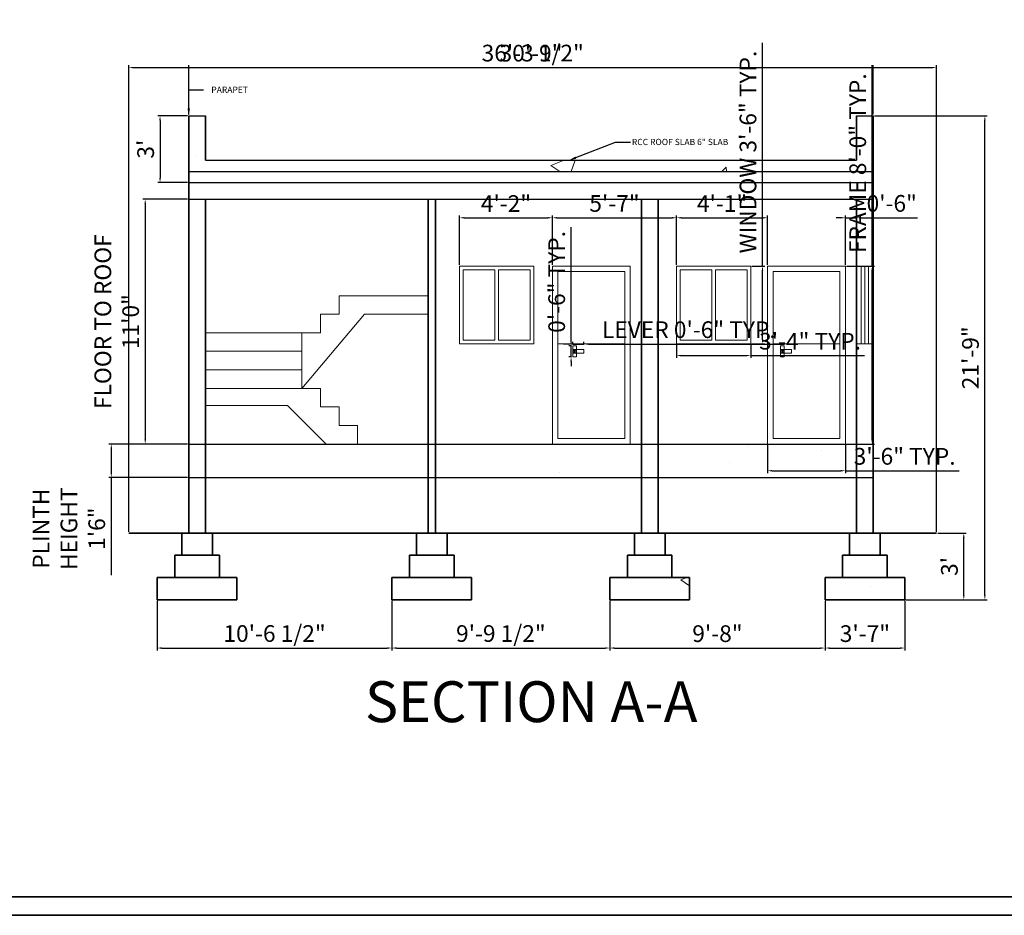
# Model space of a CAD drawing. Units: inches. Extents: x 2413 to 4117, y 1127 to 2321.
# Tile 2 of 5: x 2993 to 3524, y 1127 to 1610. Entities that reach past the tile are written whole.
import ezdxf
from ezdxf import colors
from ezdxf.entities.mleader import LeaderData, LeaderLine
from ezdxf.math import Vec2, Vec3

# ---------------------------------------------------------------- set-up
doc = ezdxf.new("R2010")
doc.units = ezdxf.units.IN
doc.linetypes.add('ACAD_ISO03W100', pattern=[30, 12, -18])
doc.layers.get('Defpoints').update_dxf_attribs({"linetype": 'ACAD_ISO03W100'})
for name, color, linetype, lineweight in [('A-ANNO-DIMS', 2, 'Continuous', 18), ('A-ANNO-TEXT', 7, 'Continuous', 18), ('A-ANNO-TITL', 7, 'Continuous', 30), ('A-ANNO-TTLB', 7, 'Continuous', 35), ('A-DOOR', 3, 'Continuous', 20), ('A-FLOR', 7, 'Continuous', 30), ('A-FLOR-STRS', 3, 'Continuous', 20), ('A-GLAZ', 4, 'Continuous', 18), ('A-ROOF', 7, 'Continuous', 30), ('A-SECT', 7, 'Continuous', 35), ('S-FNDN', 1, 'Continuous', 35), ('S-SECT-PATT', 252, 'Continuous', 13)]:
    doc.layers.add(name, color=color, linetype=linetype, lineweight=lineweight)
doc.styles.get("Standard").update_dxf_attribs({"font": 'arial.ttf'})
doc.dimstyles.new('ISO-25', dxfattribs={"dimtxt": 9, "dimasz": 2.5, "dimexe": 1.25, "dimexo": 0.625, "dimgap": 2, "dimtad": 1, "dimdec": 1, "dimlunit": 4, "dimtxsty": 'Standard', "dimcen": 2.5, "dimazin": 0, "dimtfac": 1, "dimtdec": 1, "dimtmove": 0, "dimatfit": 3, "dimfxl": 1, "dimarcsym": 0})

# ---------------------------------------------------------------- blocks, each defined once
blk = doc.blocks.new('*D1')
at = {"layer": 'A-ANNO-DIMS', "color": 0, "lineweight": -2, "transparency": 16777216}
for p, q in [((3083.32, 1513.03), (3059.22, 1513.03)), ((3060.47, 1510.53), (3060.47, 1383.53)), ((3083.32, 1381.03), (3059.22, 1381.03))]:
    blk.add_line(p, q, dxfattribs=at)
at = {"layer": 'A-ANNO-DIMS', "color": 0, "transparency": 16777216}
for points in [[(3060.06, 1510.53), (3060.89, 1510.53), (3060.47, 1513.03)], [(3060.06, 1383.53), (3060.89, 1383.53), (3060.47, 1381.03)]]:
    blk.add_solid(points, dxfattribs=at)
at = {"layer": 'Defpoints', "color": 0, "transparency": 16777216}
for p in [(3083.95, 1513.03), (3060.47, 1381.03), (3083.95, 1381.03)]:
    blk.add_point(p, dxfattribs=at)
at = {"layer": 'A-ANNO-DIMS', "color": 0, "transparency": 16777216, "insert": (3046.3, 1447.03), "char_height": 9, "attachment_point": 5, "rotation": 90}
blk.add_mtext('FLOOR TO ROOF\\P11\'0"', dxfattribs=at)
blk = doc.blocks.new('*D2')
at = {"layer": 'A-ANNO-DIMS', "color": 0, "lineweight": -2, "transparency": 16777216}
for p, q in [((3083.32, 1558.03), (3067.22, 1558.03)), ((3068.47, 1555.53), (3068.47, 1524.53)), ((3083.32, 1522.03), (3067.22, 1522.03))]:
    blk.add_line(p, q, dxfattribs=at)
at = {"layer": 'A-ANNO-DIMS', "color": 0, "transparency": 16777216}
for points in [[(3068.06, 1555.53), (3068.89, 1555.53), (3068.47, 1558.03)], [(3068.06, 1524.53), (3068.89, 1524.53), (3068.47, 1522.03)]]:
    blk.add_solid(points, dxfattribs=at)
at = {"layer": 'Defpoints', "color": 0, "transparency": 16777216}
for p in [(3083.95, 1558.03), (3068.47, 1522.03), (3083.95, 1522.03)]:
    blk.add_point(p, dxfattribs=at)
at = {"layer": 'A-ANNO-DIMS', "color": 0, "transparency": 16777216, "insert": (3061.87, 1540.03), "char_height": 9, "attachment_point": 5, "rotation": 90}
blk.add_mtext("3'", dxfattribs=at)
blk = doc.blocks.new('*D3')
at = {"layer": 'A-ANNO-DIMS', "color": 0, "lineweight": -2, "transparency": 16777216}
for p, q in [((3083.32, 1381.03), (3040.94, 1381.03)), ((3042.19, 1378.53), (3042.19, 1365.53)), ((3083.32, 1363.03), (3040.94, 1363.03)), ((3042.19, 1363.03), (3042.19, 1310.29))]:
    blk.add_line(p, q, dxfattribs=at)
at = {"layer": 'A-ANNO-DIMS', "color": 0, "transparency": 16777216}
for points in [[(3041.77, 1378.53), (3042.6, 1378.53), (3042.19, 1381.03)], [(3041.77, 1365.53), (3042.6, 1365.53), (3042.19, 1363.03)]]:
    blk.add_solid(points, dxfattribs=at)
at = {"layer": 'Defpoints', "color": 0, "transparency": 16777216}
for p in [(3083.95, 1381.03), (3042.19, 1363.03), (3083.95, 1363.03)]:
    blk.add_point(p, dxfattribs=at)
at = {"layer": 'A-ANNO-DIMS', "color": 0, "transparency": 16777216, "insert": (3020.52, 1335.41), "char_height": 9, "width": 9.6125, "attachment_point": 5, "rotation": 90}
blk.add_mtext('PLINTH HEIGHT \\P1\'6"', dxfattribs=at)
blk = doc.blocks.new('*D4')
at = {"layer": 'A-ANNO-DIMS', "color": 0, "lineweight": -2, "transparency": 16777216}
for p, q in [((3487.74, 1333.03), (3503.01, 1333.03)), ((3501.76, 1299.53), (3501.76, 1330.53)), ((3470.57, 1297.03), (3503.01, 1297.03))]:
    blk.add_line(p, q, dxfattribs=at)
at = {"layer": 'A-ANNO-DIMS', "color": 0, "transparency": 16777216}
for points in [[(3501.34, 1330.53), (3502.17, 1330.53), (3501.76, 1333.03)], [(3501.34, 1299.53), (3502.17, 1299.53), (3501.76, 1297.03)]]:
    blk.add_solid(points, dxfattribs=at)
at = {"layer": 'Defpoints', "color": 0, "transparency": 16777216}
for p in [(3487.11, 1333.03), (3501.76, 1333.03), (3469.95, 1297.03)]:
    blk.add_point(p, dxfattribs=at)
at = {"layer": 'A-ANNO-DIMS', "color": 0, "transparency": 16777216, "insert": (3495.16, 1315.03), "char_height": 9, "attachment_point": 5, "rotation": 90}
blk.add_mtext("3'", dxfattribs=at)
blk = doc.blocks.new('WIN-TWINLIGHT-40x42')
for p, q in [((0, 42), (0, 0)), ((0, 42), (40, 42)), ((2, 40), (19, 40)), ((2, 40), (2, 2)), ((19, 40), (19, 2)), ((21, 40), (21, 2)), ((21, 40), (38, 40)), ((38, 40), (38, 2)), ((40, 42), (40, 0)), ((2, 2), (19, 2)), ((21, 2), (38, 2)), ((0, 0), (40, 0))]:
    blk.add_line(p, q)
blk = doc.blocks.new('DOOR-FRAMED-42x96')
for p, q in [((0, 96), (0, 0)), ((0, 96), (42, 96)), ((42, 96), (42, 0)), ((3, 93), (39, 93)), ((3, 93), (3, 3)), ((39, 93), (39, 3)), ((3, 54), (39, 54)), ((3, 3), (39, 3))]:
    blk.add_line(p, q)
blk = doc.blocks.new('DOOR-LEVER-ELEV')
for p, q in [((0, 6), (0, 0)), ((0, 6), (2, 6)), ((2, 6), (2, 0)), ((0, 4), (6, 4)), ((0, 2), (6, 2)), ((0.18, 3), (1.82, 3)), ((1, 2.18), (1, 3.82)), ((6, 4), (6, 2)), ((0, 0), (2, 0))]:
    blk.add_line(p, q)
blk.add_circle((1, 3), 0.816)
blk = doc.blocks.new('*D26')
at = {"layer": 'A-ANNO-DIMS', "color": 0, "lineweight": -2, "transparency": 16777216}
for p, q in [((3393.25, 1477.03), (3393.25, 1597.42)), ((3387.57, 1477.03), (3394.5, 1477.03)), ((3393.25, 1437.53), (3393.25, 1474.53)), ((3387.57, 1435.03), (3394.5, 1435.03))]:
    blk.add_line(p, q, dxfattribs=at)
at = {"layer": 'A-ANNO-DIMS', "color": 0, "transparency": 16777216}
for points in [[(3392.83, 1474.53), (3393.66, 1474.53), (3393.25, 1477.03)], [(3392.83, 1437.53), (3393.66, 1437.53), (3393.25, 1435.03)]]:
    blk.add_solid(points, dxfattribs=at)
at = {"layer": 'Defpoints', "color": 0, "transparency": 16777216}
for p in [(3386.95, 1477.03), (3393.25, 1477.03), (3386.95, 1435.03)]:
    blk.add_point(p, dxfattribs=at)
at = {"layer": 'A-ANNO-DIMS', "color": 0, "transparency": 16777216, "insert": (3386.59, 1538.48), "char_height": 9, "attachment_point": 5, "rotation": 90}
blk.add_mtext('WINDOW 3\'-6" TYP.', dxfattribs=at)
blk = doc.blocks.new('*D27')
at = {"layer": 'A-ANNO-DIMS', "color": 0, "lineweight": -2, "transparency": 16777216}
for p, q in [((3346.95, 1434.41), (3346.95, 1427.48)), ((3386.95, 1434.41), (3386.95, 1427.48)), ((3349.45, 1428.73), (3384.45, 1428.73)), ((3386.95, 1428.73), (3448.3, 1428.73))]:
    blk.add_line(p, q, dxfattribs=at)
at = {"layer": 'A-ANNO-DIMS', "color": 0, "transparency": 16777216}
for points in [[(3349.45, 1429.15), (3349.45, 1428.32), (3346.95, 1428.73)], [(3384.45, 1429.15), (3384.45, 1428.32), (3386.95, 1428.73)]]:
    blk.add_solid(points, dxfattribs=at)
at = {"layer": 'Defpoints', "color": 0, "transparency": 16777216}
for p in [(3346.95, 1435.03), (3386.95, 1435.03), (3386.95, 1428.73)]:
    blk.add_point(p, dxfattribs=at)
at = {"layer": 'A-ANNO-DIMS', "color": 0, "transparency": 16777216, "insert": (3418.87, 1435.33), "char_height": 9, "attachment_point": 5}
blk.add_mtext('3\'-4" TYP.', dxfattribs=at)
blk = doc.blocks.new('*D28')
at = {"layer": 'A-ANNO-DIMS', "color": 0, "lineweight": -2, "transparency": 16777216}
for p, q in [((3452.35, 1477.03), (3452.35, 1585.38)), ((3438.57, 1477.03), (3453.6, 1477.03)), ((3452.35, 1383.53), (3452.35, 1474.53)), ((3438.57, 1381.03), (3453.6, 1381.03))]:
    blk.add_line(p, q, dxfattribs=at)
at = {"layer": 'A-ANNO-DIMS', "color": 0, "transparency": 16777216}
for points in [[(3451.93, 1474.53), (3452.76, 1474.53), (3452.35, 1477.03)], [(3451.93, 1383.53), (3452.76, 1383.53), (3452.35, 1381.03)]]:
    blk.add_solid(points, dxfattribs=at)
at = {"layer": 'Defpoints', "color": 0, "transparency": 16777216}
for p in [(3437.95, 1477.03), (3452.35, 1477.03), (3437.95, 1381.03)]:
    blk.add_point(p, dxfattribs=at)
at = {"layer": 'A-ANNO-DIMS', "color": 0, "transparency": 16777216, "insert": (3445.75, 1532.46), "char_height": 9, "attachment_point": 5, "rotation": 90}
blk.add_mtext('FRAME 8\'-0" TYP.', dxfattribs=at)
blk = doc.blocks.new('*D29')
at = {"layer": 'A-ANNO-DIMS', "color": 0, "lineweight": -2, "transparency": 16777216}
for p, q in [((3395.95, 1380.41), (3395.95, 1365.38)), ((3437.95, 1380.41), (3437.95, 1365.38)), ((3398.45, 1366.63), (3435.45, 1366.63)), ((3437.95, 1366.63), (3499.3, 1366.63))]:
    blk.add_line(p, q, dxfattribs=at)
at = {"layer": 'A-ANNO-DIMS', "color": 0, "transparency": 16777216}
for points in [[(3398.45, 1367.05), (3398.45, 1366.22), (3395.95, 1366.63)], [(3435.45, 1367.05), (3435.45, 1366.22), (3437.95, 1366.63)]]:
    blk.add_solid(points, dxfattribs=at)
at = {"layer": 'Defpoints', "color": 0, "transparency": 16777216}
for p in [(3395.95, 1381.03), (3437.95, 1381.03), (3437.95, 1366.63)]:
    blk.add_point(p, dxfattribs=at)
at = {"layer": 'A-ANNO-DIMS', "color": 0, "transparency": 16777216, "insert": (3469.87, 1373.23), "char_height": 9, "attachment_point": 5}
blk.add_mtext('3\'-6" TYP.', dxfattribs=at)
blk = doc.blocks.new('*D30')
at = {"layer": 'A-ANNO-DIMS', "color": 0, "lineweight": -2, "transparency": 16777216}
for p, q in [((3288.45, 1434.93), (3285.95, 1434.93)), ((3290.95, 1434.66), (3290.95, 1436.18)), ((3290.95, 1434.93), (3296.95, 1434.93)), ((3296.95, 1434.66), (3296.95, 1436.18)), ((3299.45, 1434.93), (3405.13, 1434.93))]:
    blk.add_line(p, q, dxfattribs=at)
at = {"layer": 'A-ANNO-DIMS', "color": 0, "transparency": 16777216}
for points in [[(3288.45, 1435.35), (3288.45, 1434.52), (3290.95, 1434.93)], [(3299.45, 1435.35), (3299.45, 1434.52), (3296.95, 1434.93)]]:
    blk.add_solid(points, dxfattribs=at)
at = {"layer": 'Defpoints', "color": 0, "transparency": 16777216}
for p in [(3290.95, 1434.03), (3296.95, 1434.93), (3296.95, 1434.03)]:
    blk.add_point(p, dxfattribs=at)
at = {"layer": 'A-ANNO-DIMS', "color": 0, "transparency": 16777216, "insert": (3353.54, 1441.53), "char_height": 9, "attachment_point": 5}
blk.add_mtext('LEVER 0\'-6" TYP.', dxfattribs=at)
blk = doc.blocks.new('*D31')
at = {"layer": 'A-ANNO-DIMS', "color": 0, "lineweight": -2, "transparency": 16777216}
for p, q in [((3290.05, 1436.53), (3290.05, 1497.89)), ((3290.32, 1434.03), (3288.8, 1434.03)), ((3290.05, 1428.03), (3290.05, 1434.03)), ((3290.32, 1428.03), (3288.8, 1428.03)), ((3290.05, 1425.53), (3290.05, 1423.03))]:
    blk.add_line(p, q, dxfattribs=at)
at = {"layer": 'A-ANNO-DIMS', "color": 0, "transparency": 16777216}
for points in [[(3289.63, 1436.53), (3290.46, 1436.53), (3290.05, 1434.03)], [(3289.63, 1425.53), (3290.46, 1425.53), (3290.05, 1428.03)]]:
    blk.add_solid(points, dxfattribs=at)
at = {"layer": 'Defpoints', "color": 0, "transparency": 16777216}
for p in [(3290.05, 1434.03), (3290.95, 1434.03), (3290.95, 1428.03)]:
    blk.add_point(p, dxfattribs=at)
at = {"layer": 'A-ANNO-DIMS', "color": 0, "transparency": 16777216, "insert": (3283.45, 1468.46), "char_height": 9, "attachment_point": 5, "rotation": 90}
blk.add_mtext('0\'-6" TYP.', dxfattribs=at)
blk = doc.blocks.new('*D77')
at = {"layer": 'A-ANNO-DIMS', "color": 0, "lineweight": -2, "transparency": 16777216}
for p, q in [((3051.65, 1333.66), (3051.65, 1585.28)), ((3054.15, 1584.03), (3484.61, 1584.03)), ((3487.11, 1333.66), (3487.11, 1585.28))]:
    blk.add_line(p, q, dxfattribs=at)
at = {"layer": 'A-ANNO-DIMS', "color": 0, "transparency": 16777216}
for points in [[(3054.15, 1584.45), (3054.15, 1583.62), (3051.65, 1584.03)], [(3484.61, 1584.45), (3484.61, 1583.62), (3487.11, 1584.03)]]:
    blk.add_solid(points, dxfattribs=at)
at = {"layer": 'Defpoints', "color": 0, "transparency": 16777216}
for p in [(3487.11, 1584.03), (3051.65, 1333.03), (3487.11, 1333.03)]:
    blk.add_point(p, dxfattribs=at)
at = {"layer": 'A-ANNO-DIMS', "color": 0, "transparency": 16777216, "insert": (3269.38, 1590.69), "char_height": 9, "attachment_point": 5}
blk.add_mtext('36\'-3 1/2"', dxfattribs=at)
blk = doc.blocks.new('*D78')
at = {"layer": 'A-ANNO-DIMS', "color": 0, "lineweight": -2, "transparency": 16777216}
for p, q in [((3453.57, 1558.03), (3514.36, 1558.03)), ((3513.11, 1299.53), (3513.11, 1555.53)), ((3470.57, 1297.03), (3514.36, 1297.03))]:
    blk.add_line(p, q, dxfattribs=at)
at = {"layer": 'A-ANNO-DIMS', "color": 0, "transparency": 16777216}
for points in [[(3512.7, 1555.53), (3513.53, 1555.53), (3513.11, 1558.03)], [(3512.7, 1299.53), (3513.53, 1299.53), (3513.11, 1297.03)]]:
    blk.add_solid(points, dxfattribs=at)
at = {"layer": 'Defpoints', "color": 0, "transparency": 16777216}
for p in [(3452.95, 1558.03), (3513.11, 1558.03), (3469.95, 1297.03)]:
    blk.add_point(p, dxfattribs=at)
at = {"layer": 'A-ANNO-DIMS', "color": 0, "transparency": 16777216, "insert": (3506.52, 1427.53), "char_height": 9, "attachment_point": 5, "rotation": 90}
blk.add_mtext('21\'-9"', dxfattribs=at)
blk = doc.blocks.new('*D79')
at = {"layer": 'A-ANNO-DIMS', "color": 0, "lineweight": -2, "transparency": 16777216}
for p, q in [((3066.95, 1296.41), (3066.95, 1269.78)), ((3193.45, 1296.41), (3193.45, 1269.78)), ((3069.45, 1271.03), (3190.95, 1271.03))]:
    blk.add_line(p, q, dxfattribs=at)
at = {"layer": 'A-ANNO-DIMS', "color": 0, "transparency": 16777216}
for points in [[(3069.45, 1271.45), (3069.45, 1270.62), (3066.95, 1271.03)], [(3190.95, 1271.45), (3190.95, 1270.62), (3193.45, 1271.03)]]:
    blk.add_solid(points, dxfattribs=at)
at = {"layer": 'Defpoints', "color": 0, "transparency": 16777216}
for p in [(3066.95, 1297.03), (3193.45, 1297.03), (3193.45, 1271.03)]:
    blk.add_point(p, dxfattribs=at)
at = {"layer": 'A-ANNO-DIMS', "color": 0, "transparency": 16777216, "insert": (3130.2, 1277.69), "char_height": 9, "attachment_point": 5}
blk.add_mtext('10\'-6 1/2"', dxfattribs=at)
blk = doc.blocks.new('*D80')
at = {"layer": 'A-ANNO-DIMS', "color": 0, "lineweight": -2, "transparency": 16777216}
for p, q in [((3193.45, 1296.41), (3193.45, 1269.78)), ((3310.95, 1296.41), (3310.95, 1269.78)), ((3195.95, 1271.03), (3308.45, 1271.03))]:
    blk.add_line(p, q, dxfattribs=at)
at = {"layer": 'A-ANNO-DIMS', "color": 0, "transparency": 16777216}
for points in [[(3195.95, 1271.45), (3195.95, 1270.62), (3193.45, 1271.03)], [(3308.45, 1271.45), (3308.45, 1270.62), (3310.95, 1271.03)]]:
    blk.add_solid(points, dxfattribs=at)
at = {"layer": 'Defpoints', "color": 0, "transparency": 16777216}
for p in [(3193.45, 1297.03), (3310.95, 1297.03), (3310.95, 1271.03)]:
    blk.add_point(p, dxfattribs=at)
at = {"layer": 'A-ANNO-DIMS', "color": 0, "transparency": 16777216, "insert": (3252.2, 1277.69), "char_height": 9, "attachment_point": 5}
blk.add_mtext('9\'-9 1/2"', dxfattribs=at)
blk = doc.blocks.new('*D81')
at = {"layer": 'A-ANNO-DIMS', "color": 0, "lineweight": -2, "transparency": 16777216}
for p, q in [((3310.95, 1296.41), (3310.95, 1269.78)), ((3426.95, 1296.41), (3426.95, 1269.78)), ((3313.45, 1271.03), (3424.45, 1271.03))]:
    blk.add_line(p, q, dxfattribs=at)
at = {"layer": 'A-ANNO-DIMS', "color": 0, "transparency": 16777216}
for points in [[(3313.45, 1271.45), (3313.45, 1270.62), (3310.95, 1271.03)], [(3424.45, 1271.45), (3424.45, 1270.62), (3426.95, 1271.03)]]:
    blk.add_solid(points, dxfattribs=at)
at = {"layer": 'Defpoints', "color": 0, "transparency": 16777216}
for p in [(3310.95, 1297.03), (3426.95, 1297.03), (3426.95, 1271.03)]:
    blk.add_point(p, dxfattribs=at)
at = {"layer": 'A-ANNO-DIMS', "color": 0, "transparency": 16777216, "insert": (3368.95, 1277.63), "char_height": 9, "attachment_point": 5}
blk.add_mtext('9\'-8"', dxfattribs=at)
blk = doc.blocks.new('*D82')
at = {"layer": 'A-ANNO-DIMS', "color": 0, "lineweight": -2, "transparency": 16777216}
for p, q in [((3426.95, 1296.41), (3426.95, 1269.78)), ((3469.95, 1296.41), (3469.95, 1269.78)), ((3429.45, 1271.03), (3467.45, 1271.03))]:
    blk.add_line(p, q, dxfattribs=at)
at = {"layer": 'A-ANNO-DIMS', "color": 0, "transparency": 16777216}
for points in [[(3429.45, 1271.45), (3429.45, 1270.62), (3426.95, 1271.03)], [(3467.45, 1271.45), (3467.45, 1270.62), (3469.95, 1271.03)]]:
    blk.add_solid(points, dxfattribs=at)
at = {"layer": 'Defpoints', "color": 0, "transparency": 16777216}
for p in [(3426.95, 1297.03), (3469.95, 1297.03), (3469.95, 1271.03)]:
    blk.add_point(p, dxfattribs=at)
at = {"layer": 'A-ANNO-DIMS', "color": 0, "transparency": 16777216, "insert": (3448.45, 1277.63), "char_height": 9, "attachment_point": 5}
blk.add_mtext('3\'-7"', dxfattribs=at)
blk = doc.blocks.new('*D83')
at = {"layer": 'A-ANNO-DIMS', "color": 0, "lineweight": -2, "transparency": 16777216}
for p, q in [((3083.95, 1558.66), (3083.95, 1585.28)), ((3086.45, 1584.03), (3450.45, 1584.03)), ((3452.95, 1558.66), (3452.95, 1585.28))]:
    blk.add_line(p, q, dxfattribs=at)
at = {"layer": 'A-ANNO-DIMS', "color": 0, "transparency": 16777216}
for points in [[(3086.45, 1584.45), (3086.45, 1583.62), (3083.95, 1584.03)], [(3450.45, 1584.45), (3450.45, 1583.62), (3452.95, 1584.03)]]:
    blk.add_solid(points, dxfattribs=at)
at = {"layer": 'Defpoints', "color": 0, "transparency": 16777216}
for p in [(3452.95, 1584.03), (3083.95, 1558.03), (3452.95, 1558.03)]:
    blk.add_point(p, dxfattribs=at)
at = {"layer": 'A-ANNO-DIMS', "color": 0, "transparency": 16777216, "insert": (3268.45, 1590.63), "char_height": 9, "attachment_point": 5}
blk.add_mtext('30\'-9"', dxfattribs=at)
blk = doc.blocks.new('*D84')
at = {"layer": 'A-ANNO-DIMS', "color": 0, "lineweight": -2, "transparency": 16777216}
for p, q in [((3435.45, 1503.03), (3432.95, 1503.03)), ((3437.95, 1477.66), (3437.95, 1504.28)), ((3437.95, 1503.03), (3443.95, 1503.03)), ((3443.95, 1477.66), (3443.95, 1504.28)), ((3446.45, 1503.03), (3476.87, 1503.03))]:
    blk.add_line(p, q, dxfattribs=at)
at = {"layer": 'A-ANNO-DIMS', "color": 0, "transparency": 16777216}
for points in [[(3435.45, 1503.45), (3435.45, 1502.62), (3437.95, 1503.03)], [(3446.45, 1503.45), (3446.45, 1502.62), (3443.95, 1503.03)]]:
    blk.add_solid(points, dxfattribs=at)
at = {"layer": 'Defpoints', "color": 0, "transparency": 16777216}
for p in [(3443.95, 1503.03), (3437.95, 1477.03), (3443.95, 1477.03)]:
    blk.add_point(p, dxfattribs=at)
at = {"layer": 'A-ANNO-DIMS', "color": 0, "transparency": 16777216, "insert": (3462.91, 1509.63), "char_height": 9, "attachment_point": 5}
blk.add_mtext('0\'-6"', dxfattribs=at)
blk = doc.blocks.new('*D85')
at = {"layer": 'A-ANNO-DIMS', "color": 0, "lineweight": -2, "transparency": 16777216}
for p, q in [((3229.95, 1477.66), (3229.95, 1504.28)), ((3232.45, 1503.03), (3277.45, 1503.03)), ((3279.95, 1477.66), (3279.95, 1504.28))]:
    blk.add_line(p, q, dxfattribs=at)
at = {"layer": 'A-ANNO-DIMS', "color": 0, "transparency": 16777216}
for points in [[(3232.45, 1503.45), (3232.45, 1502.62), (3229.95, 1503.03)], [(3277.45, 1503.45), (3277.45, 1502.62), (3279.95, 1503.03)]]:
    blk.add_solid(points, dxfattribs=at)
at = {"layer": 'Defpoints', "color": 0, "transparency": 16777216}
for p in [(3279.95, 1503.03), (3229.95, 1477.03), (3279.95, 1477.03)]:
    blk.add_point(p, dxfattribs=at)
at = {"layer": 'A-ANNO-DIMS', "color": 0, "transparency": 16777216, "insert": (3254.95, 1509.55), "char_height": 9, "attachment_point": 5}
blk.add_mtext('4\'-2"', dxfattribs=at)
blk = doc.blocks.new('*D86')
at = {"layer": 'A-ANNO-DIMS', "color": 0, "lineweight": -2, "transparency": 16777216}
for p, q in [((3279.95, 1477.66), (3279.95, 1504.28)), ((3282.45, 1503.03), (3344.45, 1503.03)), ((3346.95, 1477.66), (3346.95, 1504.28))]:
    blk.add_line(p, q, dxfattribs=at)
at = {"layer": 'A-ANNO-DIMS', "color": 0, "transparency": 16777216}
for points in [[(3282.45, 1503.45), (3282.45, 1502.62), (3279.95, 1503.03)], [(3344.45, 1503.45), (3344.45, 1502.62), (3346.95, 1503.03)]]:
    blk.add_solid(points, dxfattribs=at)
at = {"layer": 'Defpoints', "color": 0, "transparency": 16777216}
for p in [(3346.95, 1503.03), (3279.95, 1477.03), (3346.95, 1477.03)]:
    blk.add_point(p, dxfattribs=at)
at = {"layer": 'A-ANNO-DIMS', "color": 0, "transparency": 16777216, "insert": (3313.45, 1509.61), "char_height": 9, "attachment_point": 5}
blk.add_mtext('5\'-7"', dxfattribs=at)
blk = doc.blocks.new('*D87')
at = {"layer": 'A-ANNO-DIMS', "color": 0, "lineweight": -2, "transparency": 16777216}
for p, q in [((3346.95, 1477.66), (3346.95, 1504.28)), ((3349.45, 1503.03), (3393.45, 1503.03)), ((3395.95, 1477.66), (3395.95, 1504.28))]:
    blk.add_line(p, q, dxfattribs=at)
at = {"layer": 'A-ANNO-DIMS', "color": 0, "transparency": 16777216}
for points in [[(3349.45, 1503.45), (3349.45, 1502.62), (3346.95, 1503.03)], [(3393.45, 1503.45), (3393.45, 1502.62), (3395.95, 1503.03)]]:
    blk.add_solid(points, dxfattribs=at)
at = {"layer": 'Defpoints', "color": 0, "transparency": 16777216}
for p in [(3395.95, 1503.03), (3346.95, 1477.03), (3395.95, 1477.03)]:
    blk.add_point(p, dxfattribs=at)
at = {"layer": 'A-ANNO-DIMS', "color": 0, "transparency": 16777216, "insert": (3371.45, 1509.55), "char_height": 9, "attachment_point": 5}
blk.add_mtext('4\'-1"', dxfattribs=at)

msp = doc.modelspace()

# ---------------------------------------------------------------- hatches: boundary and pattern name
at = {"layer": 'S-SECT-PATT', "transparency": 33554687}
h = msp.add_hatch(dxfattribs=at)
h.set_pattern_fill('AR-CONC', color=256, scale=0.78)
h.paths.add_polyline_path([(3452.95, 1558.03), (3443.95, 1558.03), (3443.95, 1534.03), (3092.95, 1534.03), (3092.95, 1558.03), (3083.95, 1558.03), (3083.95, 1528.03), (3452.95, 1528.03)])
h.paths.add_polyline_path([(3212.95, 1381.03), (3092.95, 1381.03), (3092.95, 1363.03), (3212.95, 1363.03)])
h.paths.add_polyline_path([(3327.95, 1381.03), (3321.95, 1381.03), (3216.95, 1381.03), (3216.95, 1363.03), (3327.95, 1363.03)])
h.paths.add_polyline_path([(3443.95, 1381.03), (3437.95, 1381.03), (3336.95, 1381.03), (3336.95, 1363.03), (3443.95, 1363.03)])
h.paths.add_polyline_path([(3096.7, 1333.03), (3080.2, 1333.03), (3080.2, 1321.03), (3096.7, 1321.03)])
h.paths.add_polyline_path([(3100.45, 1321.03), (3080.2, 1321.03), (3076.45, 1321.03), (3076.45, 1309.03), (3100.45, 1309.03)])
h.paths.add_polyline_path([(3109.95, 1309.03), (3076.45, 1309.03), (3066.95, 1309.03), (3066.95, 1297.03), (3109.95, 1297.03)])
h.paths.add_polyline_path([(3223.2, 1333.03), (3206.7, 1333.03), (3206.7, 1321.03), (3223.2, 1321.03)])
h.paths.add_polyline_path([(3226.95, 1321.03), (3206.7, 1321.03), (3202.95, 1321.03), (3202.95, 1309.03), (3226.95, 1309.03)])
h.paths.add_polyline_path([(3236.45, 1309.03), (3202.95, 1309.03), (3193.45, 1309.03), (3193.45, 1297.03), (3236.45, 1297.03)])
h.paths.add_polyline_path([(3340.7, 1333.03), (3324.2, 1333.03), (3324.2, 1321.03), (3340.7, 1321.03)])
h.paths.add_polyline_path([(3344.45, 1321.03), (3324.2, 1321.03), (3320.45, 1321.03), (3320.45, 1309.03), (3344.45, 1309.03)])
h.paths.add_polyline_path([(3353.95, 1309.03), (3320.45, 1309.03), (3310.95, 1309.03), (3310.95, 1297.03), (3353.95, 1297.03)])
h.paths.add_polyline_path([(3456.7, 1333.03), (3440.2, 1333.03), (3440.2, 1321.03), (3456.7, 1321.03)])
h.paths.add_polyline_path([(3460.45, 1321.03), (3456.7, 1321.03), (3440.2, 1321.03), (3436.45, 1321.03), (3436.45, 1309.03), (3460.45, 1309.03)])
h.paths.add_polyline_path([(3469.95, 1309.03), (3460.45, 1309.03), (3436.45, 1309.03), (3426.95, 1309.03), (3426.95, 1297.03), (3469.95, 1297.03)])

# ---------------------------------------------------------------- linework, layer by layer
at = {"layer": 'A-ANNO-TTLB'}
for points in [[(2412.62, 2321.32), (4117.04, 2321.32), (4117.04, 1126.9), (2412.62, 1126.9)], [(2422.62, 2311.32), (4107.04, 2311.32), (4107.04, 1136.9), (2422.62, 1136.9)]]:
    msp.add_lwpolyline(points, close=True, dxfattribs=at)
at = {"layer": 'A-FLOR'}
for p, q in [((3083.95, 1381.03), (3321.95, 1381.03)), ((3321.95, 1381.03), (3437.95, 1381.03)), ((3437.95, 1381.03), (3452.95, 1381.03)), ((3083.95, 1363.03), (3452.95, 1363.03))]:
    msp.add_line(p, q, dxfattribs=at)
at = {"layer": 'A-FLOR-STRS'}
for p, q in [((3164.95, 1461.03), (3164.95, 1451.03)), ((3164.95, 1461.03), (3212.95, 1461.03)), ((3178.63, 1451.03), (3144.95, 1411.03)), ((3154.95, 1451.03), (3154.95, 1441.03)), ((3154.95, 1451.03), (3164.95, 1451.03)), ((3178.63, 1451.03), (3212.95, 1451.03)), ((3092.95, 1441.03), (3144.95, 1441.03)), ((3144.95, 1441.03), (3144.95, 1411.03)), ((3144.95, 1441.03), (3154.95, 1441.03)), ((3092.95, 1431.03), (3144.95, 1431.03)), ((3092.95, 1421.03), (3144.95, 1421.03)), ((3092.95, 1411.03), (3154.95, 1411.03)), ((3154.95, 1411.03), (3154.95, 1401.03)), ((3137.19, 1401.82), (3092.95, 1401.82)), ((3137.19, 1401.82), (3157.97, 1381.03)), ((3154.95, 1401.03), (3164.95, 1401.03)), ((3164.95, 1401.03), (3164.95, 1391.03)), ((3164.95, 1391.03), (3174.95, 1391.03)), ((3174.95, 1391.03), (3174.95, 1381.03))]:
    msp.add_line(p, q, dxfattribs=at)
at = {"layer": 'A-GLAZ'}
for p, q in [((3443.95, 1477.03), (3452.95, 1477.03)), ((3446.45, 1477.03), (3446.45, 1435.03)), ((3448.45, 1477.03), (3448.45, 1435.03)), ((3450.45, 1477.03), (3450.45, 1435.03)), ((3443.95, 1435.03), (3452.95, 1435.03))]:
    msp.add_line(p, q, dxfattribs=at)
at = {"layer": 'A-ROOF'}
for p, q in [((3083.95, 1558.03), (3092.95, 1558.03)), ((3443.95, 1558.03), (3452.95, 1558.03)), ((3092.95, 1534.03), (3443.95, 1534.03)), ((3083.95, 1528.03), (3452.95, 1528.03)), ((3083.95, 1522.03), (3452.95, 1522.03)), ((3083.95, 1513.03), (3216.95, 1513.03)), ((3216.95, 1513.03), (3327.95, 1513.03)), ((3327.95, 1513.03), (3452.95, 1513.03))]:
    msp.add_line(p, q, dxfattribs=at)
at = {"layer": 'A-SECT'}
for p, q in [((3083.95, 1558.03), (3083.95, 1333.03)), ((3092.95, 1558.03), (3092.95, 1534.03)), ((3443.95, 1558.03), (3443.95, 1534.03)), ((3452.95, 1558.03), (3452.95, 1333.03)), ((3092.95, 1513.03), (3092.95, 1333.03)), ((3212.95, 1513.03), (3212.95, 1333.03)), ((3216.95, 1513.03), (3216.95, 1333.03)), ((3327.95, 1513.03), (3327.95, 1333.03)), ((3336.95, 1513.03), (3336.95, 1333.03)), ((3443.95, 1513.03), (3443.95, 1333.03))]:
    msp.add_line(p, q, dxfattribs=at)
at = {"layer": 'S-FNDN'}
for p, q in [((3051.65, 1333.03), (3487.11, 1333.03)), ((3080.2, 1333.03), (3080.2, 1321.03)), ((3096.7, 1333.03), (3096.7, 1321.03)), ((3206.7, 1333.03), (3206.7, 1321.03)), ((3223.2, 1333.03), (3223.2, 1321.03)), ((3324.2, 1333.03), (3324.2, 1321.03)), ((3340.7, 1333.03), (3340.7, 1321.03)), ((3440.2, 1333.03), (3440.2, 1321.03)), ((3456.7, 1333.03), (3456.7, 1321.03)), ((3076.45, 1321.03), (3080.2, 1321.03)), ((3076.45, 1321.03), (3076.45, 1309.03)), ((3080.2, 1321.03), (3100.45, 1321.03)), ((3100.45, 1321.03), (3100.45, 1309.03)), ((3202.95, 1321.03), (3202.95, 1309.03)), ((3202.95, 1321.03), (3206.7, 1321.03)), ((3206.7, 1321.03), (3226.95, 1321.03)), ((3226.95, 1321.03), (3226.95, 1309.03)), ((3320.45, 1321.03), (3320.45, 1309.03)), ((3320.45, 1321.03), (3324.2, 1321.03)), ((3324.2, 1321.03), (3344.45, 1321.03)), ((3344.45, 1321.03), (3344.45, 1309.03)), ((3436.45, 1321.03), (3436.45, 1309.03)), ((3436.45, 1321.03), (3456.7, 1321.03)), ((3456.7, 1321.03), (3460.45, 1321.03)), ((3460.45, 1321.03), (3460.45, 1309.03)), ((3066.95, 1309.03), (3076.45, 1309.03)), ((3066.95, 1309.03), (3066.95, 1297.03)), ((3076.45, 1309.03), (3109.95, 1309.03)), ((3109.95, 1309.03), (3109.95, 1297.03)), ((3193.45, 1309.03), (3193.45, 1297.03)), ((3193.45, 1309.03), (3202.95, 1309.03)), ((3202.95, 1309.03), (3236.45, 1309.03)), ((3236.45, 1309.03), (3236.45, 1297.03)), ((3310.95, 1309.03), (3310.95, 1297.03)), ((3310.95, 1309.03), (3320.45, 1309.03)), ((3320.45, 1309.03), (3353.95, 1309.03)), ((3353.95, 1309.03), (3353.95, 1297.03)), ((3426.95, 1309.03), (3426.95, 1297.03)), ((3426.95, 1309.03), (3460.45, 1309.03)), ((3460.45, 1309.03), (3469.95, 1309.03)), ((3469.95, 1309.03), (3469.95, 1297.03)), ((3066.95, 1297.03), (3109.95, 1297.03)), ((3193.45, 1297.03), (3236.45, 1297.03)), ((3310.95, 1297.03), (3353.95, 1297.03)), ((3426.95, 1297.03), (3469.95, 1297.03))]:
    msp.add_line(p, q, dxfattribs=at)

# ---------------------------------------------------------------- block references
at = {"layer": 'A-DOOR'}
for name, p in [('DOOR-FRAMED-42x96', (3279.95, 1381.03)), ('DOOR-FRAMED-42x96', (3395.95, 1381.03)), ('DOOR-LEVER-ELEV', (3290.95, 1428.03)), ('DOOR-LEVER-ELEV', (3402.95, 1428.03))]:
    msp.add_blockref(name, p, dxfattribs=at)
at = {"layer": 'A-GLAZ'}
for p in [(3229.95, 1435.03), (3346.95, 1435.03)]:
    msp.add_blockref('WIN-TWINLIGHT-40x42', p, dxfattribs=at)

# ---------------------------------------------------------------- texts
at = {"layer": 'A-ANNO-TEXT'}
for s, height, p in [('PARAPET', 3.367, (3096.1, 1570.41)), ('RCC ROOF SLAB 6" SLAB', 3.3674, (3322.82, 1542.24))]:
    msp.add_text(s, height=height, dxfattribs=at).set_placement(p)
at = {"layer": 'A-ANNO-TITL'}
msp.add_text('SECTION A-A', height=22.0248, dxfattribs=at).set_placement((3178.92, 1231.07))

# ---------------------------------------------------------------- dimensions: what is measured, and where the dimension line sits
at = {"layer": 'A-ANNO-DIMS'}
for base, p1, p2, picture, middle in [((3487.11, 1584.03), (3051.65, 1333.03), (3487.11, 1333.03), '*D77', (3269.38, 1590.69)), ((3452.95, 1584.03), (3083.95, 1558.03), (3452.95, 1558.03), '*D83', (3268.45, 1590.63)), ((3279.95, 1503.03), (3229.95, 1477.03), (3279.95, 1477.03), '*D85', (3254.95, 1509.55)), ((3346.95, 1503.03), (3279.95, 1477.03), (3346.95, 1477.03), '*D86', (3313.45, 1509.61)), ((3443.95, 1503.03), (3437.95, 1477.03), (3443.95, 1477.03), '*D84', (3462.91, 1509.63)), ((3193.45, 1271.03), (3066.95, 1297.03), (3193.45, 1297.03), '*D79', (3130.2, 1277.69)), ((3310.95, 1271.03), (3193.45, 1297.03), (3310.95, 1297.03), '*D80', (3252.2, 1277.69)), ((3426.95, 1271.03), (3310.95, 1297.03), (3426.95, 1297.03), '*D81', (3368.95, 1277.63)), ((3469.95, 1271.03), (3426.95, 1297.03), (3469.95, 1297.03), '*D82', (3448.45, 1277.63))]:
    dim = msp.add_linear_dim(base=base, p1=p1, p2=p2, dimstyle='ISO-25', override={"dimdec": 1, "dimlfac": 1, "dimrnd": 0, "dimzin": 1, "dimdsep": 46, "dimlunit": 4, "dimfrac": 2}, dxfattribs=at)
    dim.commit()
    dim.dimension.update_dxf_attribs({"geometry": picture, "text_midpoint": middle})
for base, p1, p2, text, override, picture, middle in [((3393.25, 1477.03), (3386.95, 1435.03), (3386.95, 1477.03), 'WINDOW <> TYP.', {"dimdec": 1, "dimlfac": 1, "dimrnd": 0, "dimzin": 1, "dimdsep": 46, "dimlunit": 4, "dimfrac": 2}, '*D26', (3386.59, 1538.48)), ((3452.35, 1477.03), (3437.95, 1381.03), (3437.95, 1477.03), 'FRAME <> TYP.', {"dimdec": 1, "dimlfac": 1, "dimrnd": 0, "dimzin": 1, "dimdsep": 46, "dimlunit": 4, "dimfrac": 2}, '*D28', (3445.75, 1532.46)), ((3060.47, 1381.03), (3083.95, 1513.03), (3083.95, 1381.03), 'FLOOR TO ROOF\\P11\'0"', {"dimclrd": 0, "dimclre": 0, "dimclrt": 0}, '*D1', (3046.3, 1447.03)), ((3290.05, 1434.03), (3290.95, 1428.03), (3290.95, 1434.03), '<> TYP.', {"dimdec": 1, "dimlfac": 1, "dimrnd": 0, "dimzin": 1, "dimdsep": 46, "dimlunit": 4, "dimfrac": 2}, '*D31', (3283.45, 1468.46)), ((3042.19, 1363.03), (3083.95, 1381.03), (3083.95, 1363.03), 'PLINTH HEIGHT \\P1\'6"', {"dimclrd": 0, "dimclre": 0, "dimclrt": 0}, '*D3', (3020.52, 1335.41))]:
    dim = msp.add_linear_dim(base=base, p1=p1, p2=p2, angle=90, text=text, dimstyle='ISO-25', override=override, dxfattribs=at)
    dim.commit()
    dim.dimension.update_dxf_attribs({"geometry": picture, "text_midpoint": middle})
for base, p1, p2, angle, override, picture, middle in [((3068.47, 1522.03), (3083.95, 1558.03), (3083.95, 1522.03), 90, {"dimclrd": 0, "dimclre": 0, "dimclrt": 0}, '*D2', (3061.87, 1540.03)), ((3513.11, 1558.03), (3469.95, 1297.03), (3452.95, 1558.03), 90, {"dimdec": 1, "dimlfac": 1, "dimrnd": 0, "dimzin": 1, "dimdsep": 46, "dimlunit": 4, "dimfrac": 2}, '*D78', (3506.52, 1427.53)), ((3395.95, 1503.03), (3346.95, 1477.03), (3395.95, 1477.03), 0, {"dimdec": 1, "dimlfac": 1, "dimrnd": 0, "dimzin": 1, "dimdsep": 46, "dimlunit": 4, "dimfrac": 2}, '*D87', (3371.45, 1509.55)), ((3501.76, 1333.03), (3469.95, 1297.03), (3487.11, 1333.03), 90, {"dimclrd": 0, "dimclre": 0, "dimclrt": 0}, '*D4', (3495.16, 1315.03))]:
    dim = msp.add_linear_dim(base=base, p1=p1, p2=p2, angle=angle, dimstyle='ISO-25', override=override, dxfattribs=at)
    dim.commit()
    dim.dimension.update_dxf_attribs({"geometry": picture, "text_midpoint": middle})
for base, p1, p2, text, picture, middle in [((3296.95, 1434.93), (3290.95, 1434.03), (3296.95, 1434.03), 'LEVER <> TYP.', '*D30', (3353.54, 1441.53)), ((3386.95, 1428.73), (3346.95, 1435.03), (3386.95, 1435.03), '<> TYP.', '*D27', (3418.87, 1435.33)), ((3437.95, 1366.63), (3395.95, 1381.03), (3437.95, 1381.03), '<> TYP.', '*D29', (3469.87, 1373.23))]:
    dim = msp.add_linear_dim(base=base, p1=p1, p2=p2, text=text, dimstyle='ISO-25', override={"dimdec": 1, "dimlfac": 1, "dimrnd": 0, "dimzin": 1, "dimdsep": 46, "dimlunit": 4, "dimfrac": 2}, dxfattribs=at)
    dim.commit()
    dim.dimension.update_dxf_attribs({"geometry": picture, "text_midpoint": middle})

# ---------------------------------------------------------------- leaders
at = {"layer": 'A-ANNO-TEXT'}
ml = msp.add_multileader_mtext('Standard', dxfattribs=at)
ml.set_content('', color=256)
ml.set_leader_properties()
ml.build(insert=Vec2(0, 0))
ctx = ml.context
ctx.base_point, ctx.plane_origin = Vec3(3091.95, 1572.06), Vec3(3083.95, 1558.03)
notes = []
notes.append((ctx, [(0, (1, 1, 0), (3083.95, 1572.06), (1, 0), 8, [(0, [(3083.95, 1558.03)], 0, [])])]))
ctx.mtext.insert, ctx.mtext.flow_direction = Vec3(3093.95, 1574.06), 5
ml = msp.add_multileader_mtext('Standard', dxfattribs=at)
ml.set_content('', color=256)
ml.set_leader_properties()
ml.build(insert=Vec2(0, 0))
ctx = ml.context
ctx.base_point, ctx.plane_origin = Vec3(3322.08, 1543.73), Vec3(3288.94, 1534.03)
notes.append((ctx, [(0, (1, 1, 0), (3314.08, 1543.73), (1, 0), 8, [(0, [(3288.94, 1534.03)], 0, [])])]))
ctx.mtext.insert, ctx.mtext.flow_direction = Vec3(3324.08, 1545.73), 5
for ctx, leaders in notes:
    for number, flags, end, landing, length, lines in leaders:
        leader = LeaderData()
        leader.index, (leader.has_last_leader_line, leader.has_dogleg_vector, leader.attachment_direction) = number, flags
        leader.last_leader_point, leader.dogleg_vector, leader.dogleg_length = Vec3(end), Vec3(landing), length
        for number, points, colour, breaks in lines:
            line = LeaderLine()
            line.index, line.vertices, line.color, line.breaks = number, Vec3.list(points), colors.encode_raw_color(colour), breaks
            leader.lines.append(line)
        ctx.leaders.append(leader)

doc.saveas('drawing.dxf')
